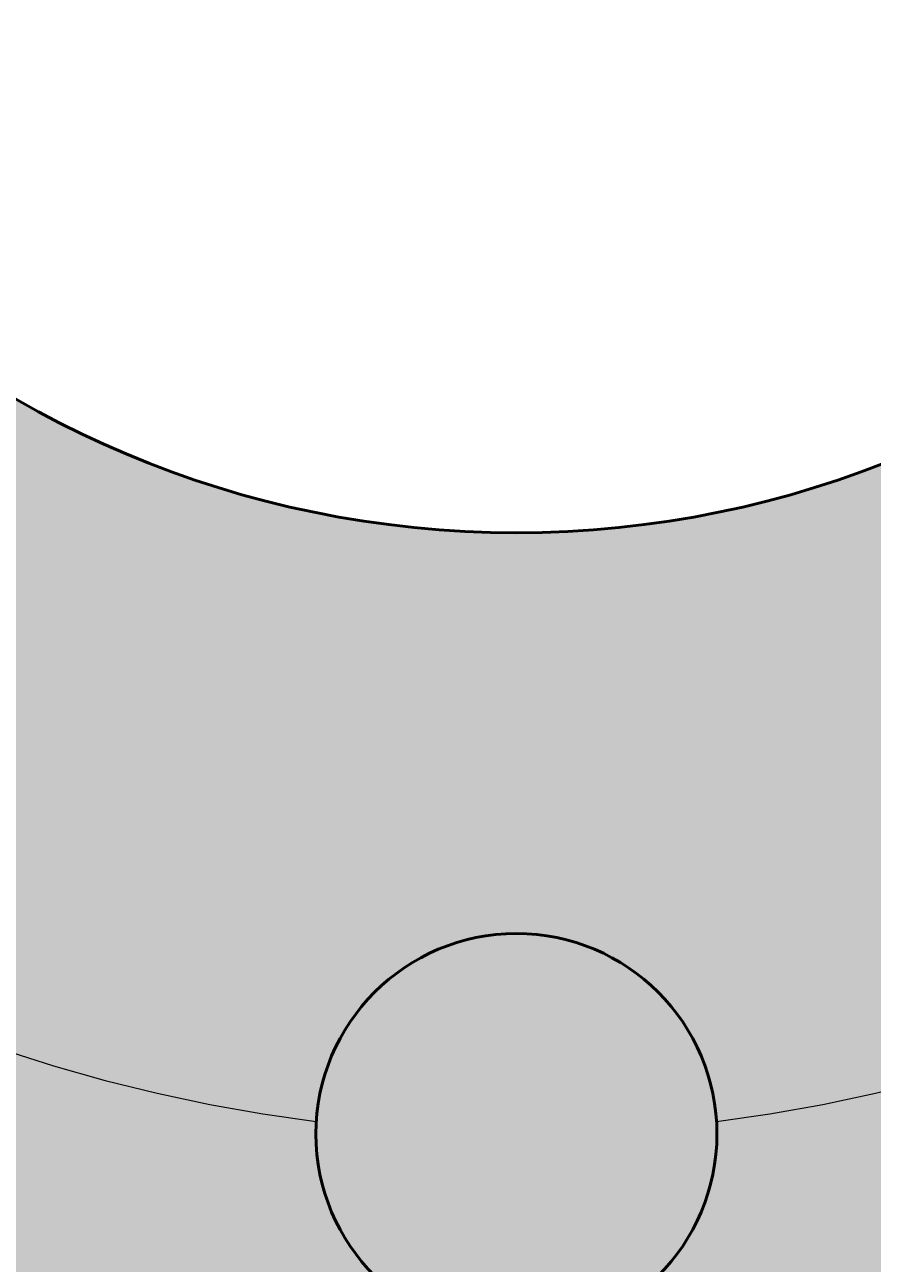
# Model space of a CAD drawing. Units: inches. Extents: x 139261 to 139415, y 52839 to 52963.
# Tile 9 of 20: x 139328 to 139349, y 52857 to 52888. Entities that reach past the tile are written whole.
import ezdxf

# ---------------------------------------------------------------- set-up
doc = ezdxf.new("R2010")
doc.units = ezdxf.units.IN
doc.header["$MEASUREMENT"] = 0
doc.linetypes.add('CENTER', pattern=[50.8, 31.75, -6.35, 6.35, -6.35])
for name, color, linetype, lineweight in [('M-CNTR', 4, 'CENTER', 18), ('M-DIMS', 2, 'Continuous', 25), ('M-HATC', 8, 'Continuous', 18), ('M-OUTL', 7, 'Continuous', 50)]:
    doc.layers.add(name, color=color, linetype=linetype, lineweight=lineweight)
doc.styles.get("Standard").update_dxf_attribs({"font": 'arial.ttf'})
doc.dimstyles.get("Standard").update_dxf_attribs({"dimtxt": 0.18, "dimasz": 0.18, "dimexe": 0.18, "dimexo": 0.0625, "dimgap": 0.09, "dimtad": 0, "dimtih": 1, "dimtoh": 1, "dimdec": 4, "dimzin": 0, "dimdsep": 46, "dimtxsty": 'Standard', "dimcen": 0.09, "dimadec": 0, "dimazin": 0, "dimtfac": 1, "dimtdec": 4, "dimtofl": 0, "dimtmove": 0, "dimatfit": 3, "dimfxl": 1, "dimtolj": 1, "dimtzin": 0, "dimarcsym": 0})

# ---------------------------------------------------------------- blocks, each defined once
blk = doc.blocks.new('*U1')
blk.add_circle((0, 0), 5)
blk = doc.blocks.new('*U2')
at = {"layer": 'M-OUTL', "color": 0, "linetype": 'ByBlock', "lineweight": -2, "transparency": 16777216, "rotation": 180}
blk.add_blockref('*U1', (139340.357, 52860.217), dxfattribs=at)
blk = doc.blocks.new('*D4')
at = {"layer": 'Defpoints', "color": 0, "transparency": 16777216}
for p in [(139373.053, 52923.26), (139307.661, 52877.175)]:
    blk.add_point(p, dxfattribs=at)
at = {"layer": 'M-DIMS', "color": 0, "lineweight": -2, "transparency": 16777216}
for p, q in [((139414.011, 52952.126), (139373.2, 52923.364)), ((139414.191, 52952.126), (139414.011, 52952.126)), ((139340.357, 52900.127), (139340.357, 52900.307)), ((139340.267, 52900.217), (139340.447, 52900.217))]:
    blk.add_line(p, q, dxfattribs=at)
blk.add_arc((139340.357, 52900.217), 40, 34.9168, 52.0771, dxfattribs=at)
at = {"layer": 'M-DIMS', "color": 0, "transparency": 16777216}
blk.add_solid([(139373.183, 52923.388), (139373.217, 52923.339), (139373.053, 52923.26)], dxfattribs=at)
at = {"layer": 'M-DIMS', "color": 0, "transparency": 16777216, "insert": (139414.822, 52952.126), "char_height": 0.18, "attachment_point": 5}
blk.add_mtext('\\A1;∅80.0000', dxfattribs=at)
blk = doc.blocks.new('*D6')
at = {"layer": 'Defpoints', "color": 0, "transparency": 16777216}
for p in [(139332.153, 52949.54), (139348.561, 52850.895)]:
    blk.add_point(p, dxfattribs=at)
at = {"layer": 'M-DIMS', "color": 0, "lineweight": -2, "transparency": 16777216}
for p, q in [((139329.787, 52962.682), (139329.967, 52962.682)), ((139329.967, 52962.682), (139332.124, 52949.717)), ((139340.357, 52900.127), (139340.357, 52900.307)), ((139340.267, 52900.217), (139340.447, 52900.217))]:
    blk.add_line(p, q, dxfattribs=at)
at = {"layer": 'M-DIMS', "color": 0, "transparency": 16777216}
blk.add_solid([(139332.153, 52949.722), (139332.094, 52949.713), (139332.153, 52949.54)], dxfattribs=at)
at = {"layer": 'M-DIMS', "color": 0, "transparency": 16777216, "insert": (139329.086, 52962.682), "char_height": 0.18, "attachment_point": 5}
blk.add_mtext('\\A1;∅100.0000', dxfattribs=at)
blk = doc.blocks.new('*D9')
at = {"layer": 'Defpoints', "color": 0, "transparency": 16777216}
for p in [(139302.054, 52932.357), (139378.659, 52868.078)]:
    blk.add_point(p, dxfattribs=at)
at = {"layer": 'M-DIMS', "color": 0, "lineweight": -2, "transparency": 16777216}
for p, q in [((139278.893, 52951.64), (139279.073, 52951.64)), ((139279.073, 52951.64), (139301.916, 52932.472)), ((139340.357, 52900.127), (139340.357, 52900.307)), ((139340.267, 52900.217), (139340.447, 52900.217))]:
    blk.add_line(p, q, dxfattribs=at)
at = {"layer": 'M-DIMS', "color": 0, "transparency": 16777216}
blk.add_solid([(139301.936, 52932.495), (139301.897, 52932.449), (139302.054, 52932.357)], dxfattribs=at)
at = {"layer": 'M-DIMS', "color": 0, "transparency": 16777216, "insert": (139278.506, 52951.64), "char_height": 0.18, "attachment_point": 5}
blk.add_mtext('\\A1;∅100', dxfattribs=at)
blk = doc.blocks.new('*D10')
at = {"layer": 'Defpoints', "color": 0, "transparency": 16777216}
for p in [(139325.07, 52937.181), (139355.644, 52863.254)]:
    blk.add_point(p, dxfattribs=at)
at = {"layer": 'M-DIMS', "color": 0, "lineweight": -2, "transparency": 16777216}
for p, q in [((139340.357, 52900.127), (139340.357, 52900.307)), ((139340.267, 52900.217), (139340.447, 52900.217)), ((139364.816, 52841.075), (139355.712, 52863.087)), ((139364.996, 52841.075), (139364.816, 52841.075))]:
    blk.add_line(p, q, dxfattribs=at)
at = {"layer": 'M-DIMS', "color": 0, "transparency": 16777216}
blk.add_solid([(139355.74, 52863.099), (139355.685, 52863.076), (139355.644, 52863.254)], dxfattribs=at)
at = {"layer": 'M-DIMS', "color": 0, "transparency": 16777216, "insert": (139365.312, 52841.075), "char_height": 0.18, "attachment_point": 5}
blk.add_mtext('\\A1;∅80', dxfattribs=at)

msp = doc.modelspace()

# ---------------------------------------------------------------- hatches: boundary and pattern name
at = {"layer": 'M-HATC'}
h = msp.add_hatch(color=256, dxfattribs=at)
h.dxf.hatch_style = 1
h.paths.add_polyline_path([(139290.35689, 52900.21749, 1), (139390.35689, 52900.21749, 1)])
h.paths.add_polyline_path([(139335.36666, 52939.90499, -0.01563646), (139335.35689, 52940.21749, -1), (139345.35689, 52940.21749, -0.01563646), (139345.34711, 52939.90499, -0.13461315), (139364.89157, 52931.80941, -0.691035), (139373.64116, 52928.50176, -0.21521822), (139371.94881, 52924.75216, -0.13461315), (139380.04439, 52905.20771, -0.43265224), (139385.35689, 52900.21749, -0.43265224), (139380.04439, 52895.22726, -0.13461315), (139371.94881, 52875.68281, -0.21521822), (139373.64116, 52871.93321, -0.691035), (139364.89157, 52868.62556, -0.13461315), (139345.34711, 52860.52999, -0.01563646), (139345.35689, 52860.21749, -1), (139335.35689, 52860.21749, -0.01563646), (139335.36666, 52860.52999, -0.13461315), (139315.82221, 52868.62556, -0.691035), (139307.07262, 52871.93321, -0.21521822), (139308.76496, 52875.68281, -0.13461315), (139300.66939, 52895.22726, -0.43265224), (139295.35689, 52900.21749, -0.43265224), (139300.66939, 52905.20771, -0.13461315), (139308.76496, 52924.75216, -0.21521822), (139307.07262, 52928.50176, -0.691035), (139315.82221, 52931.80941, -0.13461315)], flags=16)
h.paths.add_polyline_path([(139365.35689, 52900.21749, -1), (139315.35689, 52900.21749, -1)], flags=0)
h.paths.add_polyline_path([(139323.71474, 52911.30978), (139356.99903, 52911.30978, -0.3027197), (139356.99903, 52889.12519), (139323.71474, 52889.12519, -0.3027197)], flags=0)
h.paths.add_polyline_path([(139364.89157, 52931.80941, 0.13461315), (139345.34711, 52939.90499, -0.93933644), (139335.36666, 52939.90499, 0.13461315), (139315.82221, 52931.80941, -0.18270763), (139317.07262, 52928.50176, -0.64579494), (139308.76496, 52924.75216, 0.13461315), (139300.66939, 52905.20771, -0.39601219), (139305.35689, 52900.21749, -0.39601219), (139300.66939, 52895.22726, 0.13461315), (139308.76496, 52875.68281, -0.64579494), (139317.07262, 52871.93321, -0.18270763), (139315.82221, 52868.62556, 0.13461315), (139335.36666, 52860.52999, -0.93933644), (139345.34711, 52860.52999, 0.13461315), (139364.89157, 52868.62556, -0.18270763), (139363.64116, 52871.93321, -0.64579494), (139371.94881, 52875.68281, 0.13461315), (139380.04439, 52895.22726, -0.39601219), (139375.35689, 52900.21749, -0.39601219), (139380.04439, 52905.20771, 0.13461315), (139371.94881, 52924.75216, -0.64579494), (139363.64116, 52928.50176, -0.18270763)], flags=0)
h = msp.add_hatch(color=256, dxfattribs=at)
h.dxf.hatch_style = 1
h.set_gradient(color1=(205, 105, 40), tint=1)
h.paths.add_polyline_path([(139335.35689, 52940.21749, 1), (139345.35689, 52940.21749, 1)])
h.paths.add_polyline_path([(139307.07262, 52928.50176, 1), (139317.07262, 52928.50176, 1)])
h.paths.add_polyline_path([(139295.35689, 52900.21749, 1), (139305.35689, 52900.21749, 1)])
h.paths.add_polyline_path([(139307.07262, 52871.93321, 1), (139317.07262, 52871.93321, 1)])
h.paths.add_polyline_path([(139345.35689, 52860.21749, 1), (139335.35689, 52860.21749, 1)])
h.paths.add_polyline_path([(139363.64116, 52871.93321, 1), (139373.64116, 52871.93321, 1)])
h.paths.add_polyline_path([(139375.35689, 52900.21749, 1), (139385.35689, 52900.21749, 1)])
h.paths.add_polyline_path([(139363.64116, 52928.50176, 1), (139373.64116, 52928.50176, 1)])
h = msp.add_hatch(color=256, dxfattribs=at)
h.dxf.hatch_style = 1
h.paths.add_polyline_path([(139345.34711, 52939.90499, -0.93933644), (139335.36666, 52939.90499, 0.13461315), (139315.82221, 52931.80941, -0.18270763), (139317.07262, 52928.50176, -0.64579494), (139308.76496, 52924.75216, 0.13461315), (139300.66939, 52905.20771, -0.39601219), (139305.35689, 52900.21749, -0.39601219), (139300.66939, 52895.22726, 0.13461315), (139308.76496, 52875.68281, -0.64579494), (139317.07262, 52871.93321, -0.18270763), (139315.82221, 52868.62556, 0.13461315), (139335.36666, 52860.52999, -0.93933644), (139345.34711, 52860.52999, 0.13461315), (139364.89157, 52868.62556, -0.18270763), (139363.64116, 52871.93321, -0.64579494), (139371.94881, 52875.68281, 0.13461315), (139380.04439, 52895.22726, -0.39601219), (139375.35689, 52900.21749, -0.39601219), (139380.04439, 52905.20771, 0.13461315), (139371.94881, 52924.75216, -0.64579494), (139363.64116, 52928.50176, -0.18270763), (139364.89157, 52931.80941, 0.13461315)])
h.paths.add_polyline_path([(139365.35689, 52900.21749, -1), (139315.35689, 52900.21749, -1)], flags=16)
h.paths.add_polyline_path([(139356.99903, 52911.30978, -0.3027197), (139356.99903, 52889.12519), (139323.71474, 52889.12519, -0.3027197), (139323.71474, 52911.30978)], flags=0)

# ---------------------------------------------------------------- linework, layer by layer
at = {"layer": 'M-CNTR'}
for start, end in [(232.166643, 262.833357), (277.166643, 307.833357)]:
    msp.add_arc((139340.35689, 52900.21749), 40, start, end, dxfattribs=at)
at = {"layer": 'M-OUTL'}
for radius in [50, 25]:
    msp.add_circle((139340.35689, 52900.21749), radius, dxfattribs=at)

# ---------------------------------------------------------------- block references
msp.add_blockref('*U2', (0, 0), dxfattribs=at)

# ---------------------------------------------------------------- dimensions: what is measured, and where the dimension line sits
at = {"layer": 'M-DIMS'}
for p1, p2, override, picture, middle in [((139348.56051, 52850.89507), (139332.15326, 52949.5399), {"dimclrd": 0, "dimclre": 0, "dimclrt": 0}, '*D6', (139329.08622, 52962.68242)), ((139307.66087, 52877.17469), (139373.0529, 52923.26028), {"dimclrd": 0, "dimclre": 0, "dimclrt": 0}, '*D4', (139414.82217, 52952.12585)), ((139378.65939, 52868.07845), (139302.05438, 52932.35652), {"dimdec": 0, "dimlfac": 1, "dimrnd": 0, "dimzin": 0, "dimdsep": 46, "dimlunit": 2}, '*D9', (139278.50641, 52951.63995)), ((139325.07023, 52937.18123), (139355.64354, 52863.25374), {"dimdec": 0, "dimlfac": 1, "dimrnd": 0, "dimzin": 0, "dimdsep": 46, "dimlunit": 2}, '*D10', (139365.31206, 52841.0755))]:
    dim = msp.add_diameter_dim_2p(p1=p1, p2=p2, dimstyle='Standard', override=override, dxfattribs=at)
    dim.commit()
    dim.dimension.update_dxf_attribs({"geometry": picture, "text_midpoint": middle, "dimtype": 163})

doc.saveas('drawing.dxf')
